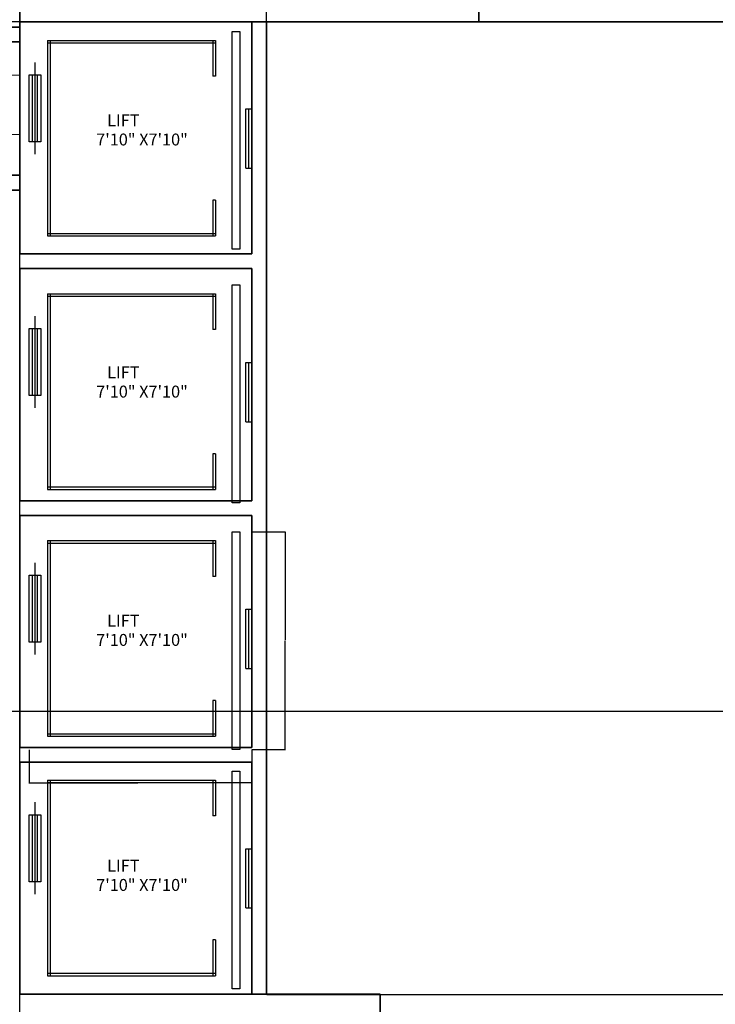
# Model space of a CAD drawing. Units: inches. Extents: x -61 to 1599, y -1316 to 257.
# Tile 95 of 204: x 545 to 826, y -565 to -166. Entities that reach past the tile are written whole.
import ezdxf

# ---------------------------------------------------------------- set-up
doc = ezdxf.new("R2010")
doc.units = ezdxf.units.IN
doc.header["$MEASUREMENT"] = 0
for name, color, linetype, lineweight in [('A-ANNO-DIMS', 2, 'Continuous', 18), ('A-AREA-IDEN', 1, 'Continuous', 18), ('A-EQPM-ELEV', 150, 'Continuous', 25), ('WALLS', 4, 'Continuous', 35), ('WINDOWS', 220, 'Continuous', 18)]:
    doc.layers.add(name, color=color, linetype=linetype, lineweight=lineweight)
doc.styles.get("Standard").update_dxf_attribs({"font": 'arial.ttf'})
doc.dimstyles.get("Standard").update_dxf_attribs({"dimtxt": 0.18, "dimasz": 0.18, "dimexe": 0.18, "dimexo": 0.0625, "dimgap": 0.09, "dimtad": 0, "dimtih": 1, "dimtoh": 1, "dimdec": 0, "dimzin": 0, "dimdsep": 46, "dimlunit": 3, "dimtxsty": 'Standard', "dimcen": 0.09, "dimadec": 0, "dimazin": 0, "dimtfac": 1, "dimtdec": 0, "dimtofl": 0, "dimtmove": 0, "dimatfit": 3, "dimfxl": 1, "dimtolj": 1, "dimtzin": 0, "dimarcsym": 0})

# ---------------------------------------------------------------- blocks, each defined once
blk = doc.blocks.new('WIN-24IN')
for p, q in [((0, 4.5), (0, 9)), ((0, 9), (0, 0)), ((24, 9), (24, 0)), ((0, 5.19), (24, 5.19)), ((0, 4.5), (24, 4.5))]:
    blk.add_line(p, q)
blk = doc.blocks.new('LIFT-PASSENGER-CAR')
for p, q in [((7.42, 84.63), (75.43, 84.63)), ((7.42, 84.63), (7.42, 5.37)), ((8.42, 84.63), (8.42, 5.37)), ((74.43, 84.63), (74.43, 70.16)), ((75.43, 84.63), (75.43, 70.16)), ((7.42, 83.63), (75.43, 83.63)), ((2.34, 70.61), (2.34, 75.61)), ((1.34, 43.45), (1.34, 70.61)), ((2.34, 43.45), (2.34, 70.61)), ((3.34, 43.45), (3.34, 70.61)), ((75.43, 70.16), (74.43, 70.16)), ((87.73, 32.82), (87.73, 56.82)), ((87.73, 56.82), (90.13, 56.82)), ((88.93, 32.82), (88.93, 56.82)), ((90.13, 32.82), (90.13, 56.82)), ((2.34, 38.45), (2.34, 43.45)), ((87.73, 32.82), (90.13, 32.82)), ((74.43, 19.85), (74.43, 5.37)), ((75.43, 19.85), (74.43, 19.85)), ((75.43, 19.85), (75.43, 5.37)), ((7.42, 6.37), (75.43, 6.37)), ((7.42, 5.37), (75.43, 5.37))]:
    blk.add_line(p, q)
for points in [[(85.24, 0), (82.13, 0), (82.13, 88.2), (85.24, 88.2)], [(4.68, 43.45), (0, 43.45), (0, 70.61), (4.68, 70.61)]]:
    blk.add_lwpolyline(points, close=True)
blk = doc.blocks.new('*D648')
at = {"layer": 'A-ANNO-DIMS', "color": 0, "lineweight": -2, "transparency": 16777216}
for p, q in [((548.58, -462.06), (548.58, -475.69)), ((638.7, -462.06), (638.7, -475.69)), ((548.76, -475.51), (592.52, -475.51)), ((638.52, -475.51), (594.76, -475.51))]:
    blk.add_line(p, q, dxfattribs=at)
at = {"layer": 'A-ANNO-DIMS', "color": 0, "transparency": 16777216}
for points in [[(548.76, -475.48), (548.76, -475.54), (548.58, -475.51)], [(638.52, -475.48), (638.52, -475.54), (638.7, -475.51)]]:
    blk.add_solid(points, dxfattribs=at)
at = {"layer": 'DEFPOINTS', "color": 0, "transparency": 16777216}
for p in [(548.58, -461.99), (638.7, -461.99), (638.7, -475.51)]:
    blk.add_point(p, dxfattribs=at)
at = {"layer": 'A-ANNO-DIMS', "color": 0, "transparency": 16777216, "insert": (593.64, -475.51), "char_height": 0.18, "attachment_point": 5}
blk.add_mtext('\\A1;LIFT CAR 90 TYP.', dxfattribs=at)
blk = doc.blocks.new('*D649')
at = {"layer": 'A-ANNO-DIMS', "color": 0, "lineweight": -2, "transparency": 16777216}
for p, q in [((638.77, -373.8), (652.4, -373.8)), ((652.22, -373.98), (652.22, -417.71)), ((652.22, -461.81), (652.22, -418.08)), ((638.77, -461.99), (652.4, -461.99))]:
    blk.add_line(p, q, dxfattribs=at)
at = {"layer": 'A-ANNO-DIMS', "color": 0, "transparency": 16777216}
for points in [[(652.19, -373.98), (652.25, -373.98), (652.22, -373.8)], [(652.19, -461.81), (652.25, -461.81), (652.22, -461.99)]]:
    blk.add_solid(points, dxfattribs=at)
at = {"layer": 'DEFPOINTS', "color": 0, "transparency": 16777216}
for p in [(638.7, -373.8), (652.22, -373.8), (638.7, -461.99)]:
    blk.add_point(p, dxfattribs=at)
at = {"layer": 'A-ANNO-DIMS', "color": 0, "transparency": 16777216, "insert": (652.22, -417.89), "char_height": 0.18, "attachment_point": 5}
blk.add_mtext('\\A1;88 TYP.', dxfattribs=at)
blk = doc.blocks.new('*D697')
at = {"layer": 'A-ANNO-DIMS', "color": 0, "lineweight": -2, "transparency": 16777216}
for p, q in [((644.7, -561.11), (644.7, 257.46)), ((644.88, 257.28), (739.94, 257.28)), ((835.52, 257.28), (740.47, 257.28)), ((835.7, -563.19), (835.7, 257.46))]:
    blk.add_line(p, q, dxfattribs=at)
at = {"layer": 'A-ANNO-DIMS', "color": 0, "transparency": 16777216}
for points in [[(644.88, 257.31), (644.88, 257.25), (644.7, 257.28)], [(835.52, 257.31), (835.52, 257.25), (835.7, 257.28)]]:
    blk.add_solid(points, dxfattribs=at)
at = {"layer": 'DEFPOINTS', "color": 0, "transparency": 16777216}
for p in [(835.7, 257.28), (644.7, -561.17), (835.7, -563.25)]:
    blk.add_point(p, dxfattribs=at)
at = {"layer": 'A-ANNO-DIMS', "color": 0, "transparency": 16777216, "insert": (740.2, 257.28), "char_height": 0.18, "attachment_point": 5}
blk.add_mtext('\\A1;191', dxfattribs=at)
blk = doc.blocks.new('*D698')
at = {"layer": 'A-ANNO-DIMS', "color": 0, "lineweight": -2, "transparency": 16777216}
for p, q in [((644.77, -167.17), (1598.48, -167.17)), ((1598.3, -167.35), (1598.3, -363.99)), ((1598.3, -560.99), (1598.3, -364.35)), ((644.77, -561.17), (1598.48, -561.17))]:
    blk.add_line(p, q, dxfattribs=at)
at = {"layer": 'A-ANNO-DIMS', "color": 0, "transparency": 16777216}
for points in [[(1598.27, -167.35), (1598.33, -167.35), (1598.3, -167.17)], [(1598.27, -560.99), (1598.33, -560.99), (1598.3, -561.17)]]:
    blk.add_solid(points, dxfattribs=at)
at = {"layer": 'DEFPOINTS', "color": 0, "transparency": 16777216}
for p in [(644.7, -167.17), (1598.3, -167.17), (644.7, -561.17)]:
    blk.add_point(p, dxfattribs=at)
at = {"layer": 'A-ANNO-DIMS', "color": 0, "transparency": 16777216, "insert": (1598.3, -364.17), "char_height": 0.18, "attachment_point": 5}
blk.add_mtext('\\A1;394', dxfattribs=at)
blk = doc.blocks.new('*D699')
at = {"layer": 'A-ANNO-DIMS', "color": 0, "lineweight": -2, "transparency": 16777216}
for p, q in [((835.64, -167.17), (-61.08, -167.17)), ((-60.9, -167.35), (-60.9, -306.73)), ((-60.9, -446.47), (-60.9, -307.09)), ((841.64, -446.65), (-61.08, -446.65))]:
    blk.add_line(p, q, dxfattribs=at)
at = {"layer": 'A-ANNO-DIMS', "color": 0, "transparency": 16777216}
for points in [[(-60.93, -167.35), (-60.87, -167.35), (-60.9, -167.17)], [(-60.93, -446.47), (-60.87, -446.47), (-60.9, -446.65)]]:
    blk.add_solid(points, dxfattribs=at)
at = {"layer": 'DEFPOINTS', "color": 0, "transparency": 16777216}
for p in [(835.7, -167.17), (-60.9, -446.65), (841.7, -446.65)]:
    blk.add_point(p, dxfattribs=at)
at = {"layer": 'A-ANNO-DIMS', "color": 0, "transparency": 16777216, "insert": (-60.9, -306.91), "char_height": 0.18, "attachment_point": 5}
blk.add_mtext('\\A1;279.5', dxfattribs=at)
blk = doc.blocks.new('*D704')
at = {"layer": 'A-ANNO-DIMS', "color": 0, "lineweight": -2, "transparency": 16777216}
for p, q in [((491.83, -616.88), (491.83, 257.46)), ((492.01, 257.28), (517.87, 257.28)), ((544.52, 257.28), (518.66, 257.28)), ((544.7, -616.88), (544.7, 257.46))]:
    blk.add_line(p, q, dxfattribs=at)
at = {"layer": 'A-ANNO-DIMS', "color": 0, "transparency": 16777216}
for points in [[(492.01, 257.31), (492.01, 257.25), (491.83, 257.28)], [(544.52, 257.31), (544.52, 257.25), (544.7, 257.28)]]:
    blk.add_solid(points, dxfattribs=at)
at = {"layer": 'DEFPOINTS', "color": 0, "transparency": 16777216}
for p in [(544.7, 257.28), (491.83, -616.94), (544.7, -616.94)]:
    blk.add_point(p, dxfattribs=at)
at = {"layer": 'A-ANNO-DIMS', "color": 0, "transparency": 16777216, "insert": (518.27, 257.28), "char_height": 0.18, "attachment_point": 5}
blk.add_mtext('\\A1;52.87', dxfattribs=at)

msp = doc.modelspace()

# ---------------------------------------------------------------- linework, layer by layer
at = {"layer": 'WALLS'}
for p, q in [((730.7028, -167.169), (730.7028, -61.169)), ((544.7028, -161.169), (544.7028, -167.169)), ((730.7028, -167.169), (544.7028, -167.169)), ((544.7028, -167.169), (544.7028, -261.169)), ((638.7028, -167.169), (638.7028, -261.169)), ((644.7028, -167.169), (644.7028, -267.169)), ((397.7028, -169.3229), (544.7028, -169.3229)), ((535.7028, -175.3229), (544.7028, -175.3229)), ((544.7028, -188.7661), (544.7028, -212.7661)), ((367.7028, -229.3229), (544.7028, -229.3229)), ((433.7028, -229.3229), (544.7028, -229.3229)), ((367.7028, -235.3229), (544.7028, -235.3229)), ((433.7028, -235.3229), (544.7028, -235.3229)), ((638.7028, -261.169), (544.7028, -261.169)), ((638.7028, -267.169), (544.7028, -267.169)), ((544.7028, -267.169), (544.7028, -361.169)), ((638.7028, -267.169), (638.7028, -361.169)), ((644.7028, -267.169), (644.7028, -367.169)), ((638.7028, -361.169), (544.7028, -361.169)), ((638.7028, -367.169), (544.7028, -367.169)), ((544.7028, -367.169), (544.7028, -461.169)), ((638.7028, -367.169), (638.7028, -461.169)), ((644.7028, -367.169), (644.7028, -467.169)), ((638.7028, -461.169), (544.7028, -461.169)), ((638.7028, -467.169), (544.7028, -467.169)), ((544.7028, -467.169), (544.7028, -561.169)), ((638.7028, -467.169), (638.7028, -561.169)), ((644.7028, -467.169), (644.7028, -561.169)), ((690.7028, -561.169), (544.7028, -561.169)), ((685.7028, -561.169), (544.7028, -561.169)), ((690.7028, -741.169), (690.7028, -561.169))]:
    msp.add_line(p, q, dxfattribs=at)

# ---------------------------------------------------------------- block references
at = {"layer": 'A-EQPM-ELEV'}
for p in [(548.575, -259.302), (548.575, -361.9923), (548.575, -461.9923), (548.575, -558.9923)]:
    msp.add_blockref('LIFT-PASSENGER-CAR', p, dxfattribs=at)
at = {"layer": 'WINDOWS', "rotation": 269.9999999999998}
msp.add_blockref('WIN-24IN', (535.7027, -188.7656), dxfattribs=at)

# ---------------------------------------------------------------- texts
at = {"layer": 'A-AREA-IDEN'}
for s, height, p in [('   LIFT', 4.8321, (575.6945, -209.5028)), ('7\'10" X7\'10"', 4.832098, (575.6945, -217.2651)), ('   LIFT', 4.8321, (575.6945, -311.6441)), ('7\'10" X7\'10"', 4.832098, (575.6945, -319.4065)), ('   LIFT', 4.8321, (575.6945, -412.2398)), ('7\'10" X7\'10"', 4.832098, (575.6945, -420.0022)), ('   LIFT', 4.8321, (575.6945, -511.5081)), ('7\'10" X7\'10"', 4.832098, (575.6945, -519.2705))]:
    msp.add_text(s, height=height, dxfattribs=at).set_placement(p)

# ---------------------------------------------------------------- dimensions: what is measured, and where the dimension line sits
at = {"layer": 'A-ANNO-DIMS'}
for base, p1, p2, override, picture, middle in [((544.7028, 257.2771), (491.8327, -616.9446), (544.7028, -616.9446), {"dimdec": 2, "dimlfac": 1, "dimrnd": 0, "dimzin": 0, "dimdsep": 46, "dimlunit": 2}, '*D704', (518.2677, 257.2771)), ((835.7028, 257.2771), (644.7028, -561.169), (835.7028, -563.2524), {"dimdec": 0, "dimlfac": 1, "dimrnd": 0, "dimzin": 0, "dimdsep": 46, "dimlunit": 2}, '*D697', (740.2028, 257.2771))]:
    dim = msp.add_linear_dim(base=base, p1=p1, p2=p2, dimstyle='Standard', override=override, dxfattribs=at)
    dim.commit()
    dim.dimension.update_dxf_attribs({"geometry": picture, "text_midpoint": middle})
for base, p1, p2, override, picture, middle in [((-60.8972, -446.6462), (835.7028, -167.169), (841.7028, -446.6462), {"dimdec": 1, "dimlfac": 1, "dimrnd": 0, "dimzin": 0, "dimdsep": 46, "dimlunit": 2}, '*D699', (-60.8972, -306.9076)), ((1598.3028, -167.169), (644.7028, -561.169), (644.7028, -167.169), {"dimdec": 0, "dimlfac": 1, "dimrnd": 0, "dimzin": 0, "dimdsep": 46, "dimlunit": 2}, '*D698', (1598.3028, -364.169))]:
    dim = msp.add_linear_dim(base=base, p1=p1, p2=p2, angle=90, dimstyle='Standard', override=override, dxfattribs=at)
    dim.commit()
    dim.dimension.update_dxf_attribs({"geometry": picture, "text_midpoint": middle})
dim = msp.add_linear_dim(base=(652.2219, -373.7964), p1=(638.7028, -461.9928), p2=(638.7028, -373.7964), angle=90, text='<> TYP.', dimstyle='Standard', override={"dimdec": 0, "dimlfac": 1, "dimrnd": 0, "dimzin": 0, "dimdsep": 46, "dimlunit": 2}, dxfattribs=at)
dim.commit()
dim.dimension.update_dxf_attribs({"geometry": '*D649', "text_midpoint": (652.2219, -417.8946)})
dim = msp.add_linear_dim(base=(638.7028, -475.5119), p1=(548.5752, -461.9928), p2=(638.7028, -461.9928), text='LIFT CAR <> TYP.', dimstyle='Standard', override={"dimdec": 0, "dimlfac": 1, "dimrnd": 0, "dimzin": 0, "dimdsep": 46, "dimlunit": 2}, dxfattribs=at)
dim.commit()
dim.dimension.update_dxf_attribs({"geometry": '*D648', "text_midpoint": (593.639, -475.5119)})

doc.saveas('drawing.dxf')
